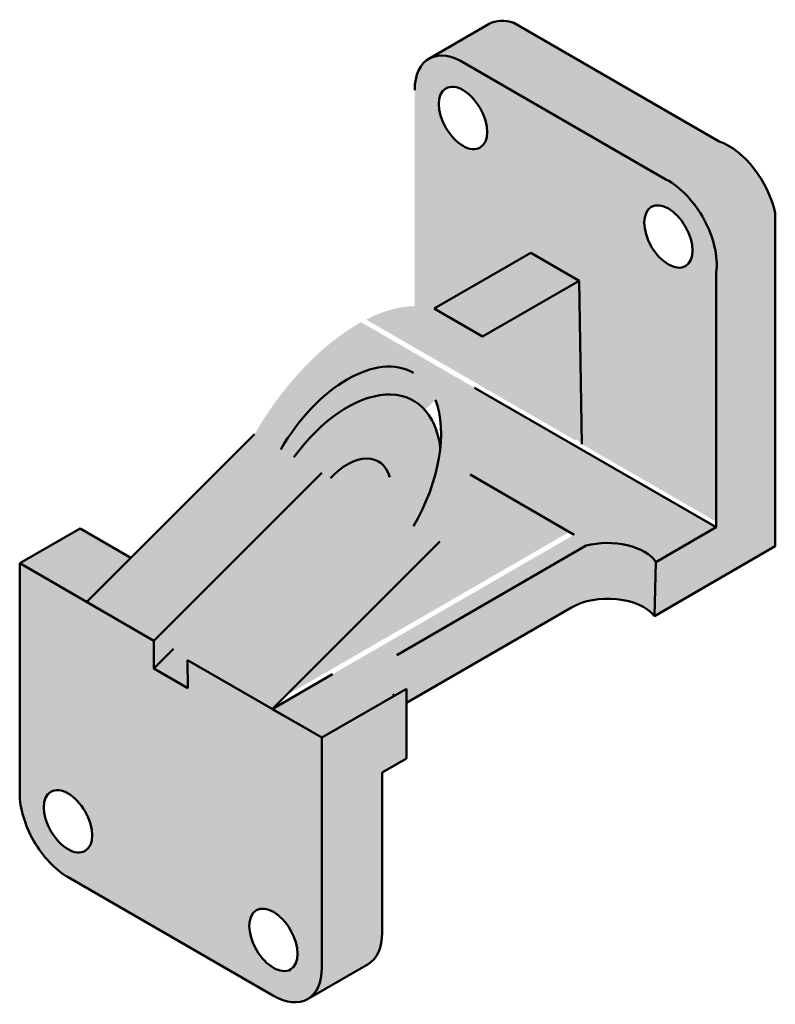
# Model space of a CAD drawing. Units: inches. Extents: x 181 to 9700, y 72 to 10161.
# Tile 1 of 2: x 181 to 452, y 72 to 425. Entities that reach past the tile are written whole.
import ezdxf

# ---------------------------------------------------------------- set-up
doc = ezdxf.new("R2010")
doc.units = ezdxf.units.IN
doc.header["$MEASUREMENT"] = 0
doc.layers.add('M-HATC', color=9, linetype='Continuous', lineweight=18)
doc.layers.add('M-OUTL', color=7, linetype='Continuous', lineweight=50)

msp = doc.modelspace()

# ---------------------------------------------------------------- hatches: boundary and pattern name
at = {"layer": 'M-HATC'}
h = msp.add_hatch(color=256, dxfattribs=at)
h.dxf.hatch_style = 1
h.paths.add_polyline_path([(289.5758214261552, 262.3998847366588), (265.5436164711371, 276.2748847366588), (205.4395400702806, 216.1708083358023), (229.4717450252987, 202.2958083358023)])
h.paths.add_polyline_path([(332.0110662115927, 237.8998847366588), (301.7001770791373, 255.3998847366588), (241.5961006782808, 195.2958083358023), (271.9069898107362, 177.7958083358023)])
edge = h.paths.add_edge_path()
edge.add_line((378.4281144762222, 241.2958083358023), (342.8085507036823, 261.8607730682951))
edge.add_ellipse((298.7773413413649, 257.0873847366588), major_axis=(-35.93948496215874, -62.24901395231655), ratio=0.5338835550983223, start_angle=450, end_angle=486.187226740073, ccw=False)
edge.add_ellipse((298.7773413413649, 257.0873847366588), major_axis=(-35.93948496215874, -62.24901395231655), ratio=0.5338835550983223, start_angle=381.6976936192442, end_angle=450, ccw=False)
edge.add_line((289.8207652336183, 195.7095837586844), (276.6390406183051, 182.5278591433712))
edge.add_line((276.6390406183051, 182.5278591433712), (291.8255740977782, 191.2958083358023))
edge.add_line((291.8255740977782, 191.2958083358023), (378.4281144762222, 241.2958083358023))
h.paths.add_polyline_path([(452.1982455472475, 236.1197151084636), (452.1982455472475, 346.5359742140326), (431.0229429833748, 334.3104075786089), (431.0229429833748, 242.9573465124921), (409.3723078887639, 230.4573465124921), (408.8969753580256, 211.1197151084636)])
edge = h.paths.add_edge_path()
edge.add_ellipse((392.1722335010851, 226.7309791545812), major_axis=(-18.37117307087383, 0), ratio=0.577350269189626, start_angle=192.224119058928, end_angle=308.65442906113)
edge.add_line((384.470166530734, 236.3604160433479), (384.470166530734, 216.3604160433479))
edge.add_ellipse((392.1722335010851, 206.7309791545811), major_axis=(-18.37117307087383, 0), ratio=0.577350269189626, start_angle=194.7034681906882, end_angle=308.65442906113003, ccw=False)
edge.add_line((408.8969753580256, 211.1197151084636), (409.3723078887639, 230.4573465124921))
edge = h.paths.add_edge_path()
edge.add_line((311.3111456829281, 155.0458083358022), (319.9713997207725, 160.0458083358023))
edge.add_line((319.9713997207725, 160.0458083358023), (319.9713997207725, 185.0458083358023))
edge.add_line((319.9713997207725, 185.0458083358023), (311.3111456829281, 180.0458083358023))
edge.add_line((311.3111456829281, 180.0458083358023), (289.6605105883172, 167.5458083358023))
edge.add_line((289.6605105883172, 167.5458083358023), (289.6605105883172, 85.04580833580225))
edge.add_ellipse((272.3400025126284, 95.04580833580229), major_axis=(12.24744871391588, -21.21320343559644), ratio=0.5773502691896262, start_angle=360.00000000000006, end_angle=390.00000000000006, ccw=False)
edge.add_line((285.6593063694593, 74.45144075550013), (306.2380863211551, 86.3326049002059))
edge.add_ellipse((293.9906376072394, 107.5458083358023), major_axis=(12.24744871391588, -21.21320343559644), ratio=0.577350269189626, start_angle=360, end_angle=390)
edge.add_line((311.3111456829281, 97.5458083358022), (311.3111456829281, 155.0458083358022))
edge = h.paths.add_edge_path()
edge.add_ellipse((361.9316820788472, 402.1604731669166), major_axis=(12.24744871391588, -21.21320343559644), ratio=0.5773502691896263, start_angle=159.0205819913284, end_angle=180)
edge.add_line((349.6842333649313, 423.3736766025129), (328.0335982703203, 410.8736766025129))
edge.add_ellipse((340.2810469842362, 389.6604731669166), major_axis=(12.24744871391588, -21.21320343559644), ratio=0.577350269189626, start_angle=152.4268374845575, end_angle=180.0000000000001, ccw=False)
edge.add_ellipse((340.2810469842362, 389.6604731669166), major_axis=(12.24744871391588, -21.21320343559644), ratio=0.577350269189626, start_angle=147.4484474656536, end_angle=152.4268374845575, ccw=False)
edge.add_line((341.1488497899605, 409.1343284863016), (413.0254035001923, 367.6363808532769))
edge.add_line((413.0254035001923, 367.6363808532769), (432.1174865026594, 381.2434445483418))
edge.add_line((432.1174865026594, 381.2434445483418), (358.5053271809825, 423.7434445483415))
edge = h.paths.add_edge_path()
edge.add_ellipse((435.5438414005244, 359.6604731669166), major_axis=(12.24744871391588, -21.21320343559644), ratio=0.577350269189626, start_angle=46.09756655575147, end_angle=159.0205819913284)
edge.add_line((432.1174865026594, 381.2434445483418), (413.0254035001923, 367.6363808532769))
edge.add_ellipse((413.8932063059135, 347.1604731669166), major_axis=(12.24744871391588, -21.21320343559644), ratio=0.5773502691896262, start_angle=37.97473599029382, end_angle=152.4268374845516, ccw=False)
edge.add_ellipse((413.8932063059135, 347.1604731669166), major_axis=(12.24744871391588, -21.21320343559644), ratio=0.5773502691896262, start_angle=23.124187939269177, end_angle=37.97473599029382, ccw=False)
edge.add_line((431.0229429833748, 334.3104075786089), (452.1982455472475, 346.5359742140326))
edge.add_line((452.1982455472475, 346.5359742140326), (452.1982455472475, 355.5381741557557))
edge = h.paths.add_edge_path()
edge.add_line((381.9139330076487, 331.3424327360183), (355.9331708941156, 316.3424327360183))
edge.add_line((355.9331708941156, 316.3424327360183), (347.2729168562712, 311.3424327360183))
edge.add_line((347.2729168562712, 311.3424327360183), (338.9373332006266, 316.1549842034574))
edge.add_ellipse((298.7773413413649, 257.0873847366588), major_axis=(-35.93948496215874, -62.24901395231655), ratio=0.5338835550983223, start_angle=516.3910297951071, end_angle=535.6085769278975)
edge.add_line((339.0824179452242, 315.9703712874247), (382.8409424408887, 272.7752374957912))
edge.add_line((382.8409424408887, 272.7752374957912), (381.9139330076487, 331.3424327360183))
edge = h.paths.add_edge_path()
edge.add_line((381.9139330076487, 331.3424327360183), (364.5934249319599, 341.3424327360183))
edge.add_line((364.5934249319599, 341.3424327360183), (338.6126628184268, 326.3424327360183))
edge.add_line((338.6126628184268, 326.3424327360183), (329.9524087805823, 321.3424327360183))
edge.add_ellipse((298.7773413413649, 257.0873847366588), major_axis=(-35.93948496215874, -62.24901395231655), ratio=0.5338835550983223, start_angle=535.8815919061803, end_angle=544.1184080938197, ccw=False)
edge.add_line((336.1655495610535, 318.417122825898), (347.2729168562712, 311.3424327360183))
edge.add_line((347.2729168562712, 311.3424327360183), (355.9331708941156, 316.3424327360183))
edge.add_line((355.9331708941156, 316.3424327360183), (381.9139330076487, 331.3424327360183))
edge = h.paths.add_edge_path()
edge.add_line((378.7961718094055, 273.1104869086883), (347.7145594960051, 291.0554641446776))
edge.add_ellipse((298.7773413413649, 257.0873847366588), major_axis=(-35.93948496215874, -62.24901395231655), ratio=0.5338835550983223, start_angle=486.187226740073, end_angle=514.7651124476778, ccw=False)
edge.add_line((342.8085507036823, 261.8607730682951), (351.059823285458, 257.0968986220499))
edge.add_line((351.059823285458, 257.0968986220499), (378.7961718094055, 273.1104869086883))
edge = h.paths.add_edge_path(flags=17)
edge.add_ellipse((298.7773413413649, 257.0873847366588), major_axis=(-35.93948496215874, -62.24901395231655), ratio=0.5338835550983223, start_angle=516.3910297951071, end_angle=535.6085769278851, ccw=False)
edge.add_line((347.6386869656112, 293.0992691705247), (380.5282226169744, 274.1104869086884))
edge.add_line((380.5282226169744, 274.1104869086884), (381.1339810930626, 274.4602217279218))
edge.add_line((381.1339810930626, 274.4602217279218), (339.0824179452354, 315.9703712874136))
h = msp.add_hatch(color=256, dxfattribs=at)
h.dxf.hatch_style = 1
edge = h.paths.add_edge_path()
edge.add_ellipse((413.8932063059135, 347.1604731669166), major_axis=(12.24744871391588, -21.21320343559644), ratio=0.5773502691896262, start_angle=37.97473599029381, end_angle=152.4268374845516)
edge.add_line((413.0254035001928, 367.6363808532767), (339.4132441785131, 410.1363808532779))
edge.add_ellipse((340.2810469842362, 389.6604731669166), major_axis=(12.24744871391588, -21.21320343559644), ratio=0.577350269189626, start_angle=152.4268374845575, end_angle=180)
edge.add_ellipse((340.2810469842362, 389.6604731669166), major_axis=(12.24744871391588, -21.21320343559644), ratio=0.577350269189626, start_angle=180, end_angle=210)
edge.add_line((322.9605389085474, 399.6604731669158), (322.9605389085474, 322.2239604497972))
edge.add_ellipse((298.7773413413649, 257.0873847366588), major_axis=(-35.93948496215874, -62.24901395231655), ratio=0.5338835550983223, start_angle=544.1184080938197, end_angle=549.6315947378079, ccw=False)
edge.add_line((329.9524087805823, 321.3424327360183), (338.6126628184268, 326.3424327360183))
edge.add_line((338.6126628184268, 326.3424327360183), (364.5934249319599, 341.3424327360183))
edge.add_line((364.5934249319599, 341.3424327360183), (381.9139330076487, 331.3424327360183))
edge.add_line((381.9139330076487, 331.3424327360183), (382.8409424408887, 272.7752374957912))
edge.add_line((382.8409424408887, 272.7752374957912), (431.0229429833748, 244.9573465124921))
edge.add_line((431.0229429833748, 244.9573465124921), (431.0229429833748, 334.3104075786089))
edge.add_ellipse((413.8932063059135, 347.1604731669166), major_axis=(12.24744871391588, -21.21320343559644), ratio=0.5773502691896262, start_angle=23.12418793926915, end_angle=37.97473599029381)
edge = h.paths.add_edge_path(flags=16)
edge.add_ellipse((413.8932063059135, 347.1604731669166), major_axis=(6.123724356957978, -10.60660171779819), ratio=0.5773502691896275, start_angle=0, end_angle=360)
edge = h.paths.add_edge_path(flags=16)
edge.add_ellipse((340.2810469842362, 389.6604731669166), major_axis=(6.123724356957978, -10.60660171779819), ratio=0.5773502691896275, start_angle=0, end_angle=360)
edge = h.paths.add_edge_path()
edge.add_line((289.6605105883172, 167.5458083358022), (241.5961006782808, 195.2958083358023))
edge.add_line((241.5961006782808, 195.2958083358023), (241.6175036323853, 185.3330109196496))
edge.add_line((241.6175036323853, 185.3330109196496), (229.4717450252987, 192.2958083358023))
edge.add_line((229.4717450252987, 192.2958083358023), (229.4717450252988, 202.2958083358023))
edge.add_line((229.4717450252988, 202.2958083358023), (181.4073351152624, 230.0458083358023))
edge.add_line((181.4073351152624, 230.0458083358023), (181.4073351152623, 147.5458083358021))
edge.add_ellipse((198.7278431909511, 137.5458083358023), major_axis=(12.24744871391588, -21.21320343559644), ratio=0.577350269189626, start_angle=210, end_angle=330.0000000000001)
edge.add_line((198.7278431909521, 117.5458083358022), (272.340002512628, 75.04580833580275))
edge.add_ellipse((272.3400025126284, 95.04580833580229), major_axis=(12.24744871391588, -21.21320343559644), ratio=0.5773502691896262, start_angle=330.0000000000001, end_angle=360)
edge.add_ellipse((272.3400025126284, 95.04580833580229), major_axis=(12.24744871391588, -21.21320343559644), ratio=0.5773502691896262, start_angle=360, end_angle=390.0000000000001)
edge.add_line((289.6605105883172, 85.04580833580206), (289.6605105883172, 167.5458083358022))
edge = h.paths.add_edge_path(flags=16)
edge.add_ellipse((272.3400025126284, 95.04580833580229), major_axis=(6.123724356957941, -10.60660171779822), ratio=0.5773502691896262, start_angle=0, end_angle=360)
edge = h.paths.add_edge_path(flags=16)
edge.add_ellipse((198.7278431909511, 137.5458083358023), major_axis=(6.123724356957941, -10.60660171779822), ratio=0.577350269189626, start_angle=0, end_angle=360)
edge = h.paths.add_edge_path()
edge.add_line((319.9713997207725, 185.0458083358023), (319.9713997207725, 180.6632076835423))
edge.add_ellipse((329.6161445207665, 189.6905531357963), major_axis=(-18.37117307087383, 0), ratio=0.5773502691896243, start_angle=403.1061845214365, end_angle=405.8946704081265)
edge.add_line((320.6448648053178, 180.4346335836542), (379.1818524443187, 214.2309791545812))
edge.add_ellipse((392.1722335010851, 206.7309791545811), major_axis=(-18.37117307087383, 0), ratio=0.577350269189626, start_angle=308.65442906113003, end_angle=330.00000000000006, ccw=False)
edge.add_line((384.470166530734, 216.3604160433479), (384.470166530734, 236.3604160433479))
edge.add_ellipse((392.1722335010851, 226.7309791545812), major_axis=(-18.37117307087383, 0), ratio=0.577350269189626, start_angle=552.224119058928, end_angle=668.65442906113, ccw=False)
edge.add_line((409.3723078887639, 230.4573465124921), (431.0229429833748, 242.9573465124921))
edge.add_line((431.0229429833748, 242.9573465124921), (381.1479140261116, 271.7527079068085))
edge.add_line((381.1479140261116, 271.7527079068085), (354.0364540342908, 255.3783400579332))
edge.add_line((354.0364540342908, 255.3783400579332), (380.160165283791, 240.2958083358022))
edge.add_line((380.160165283791, 240.2958083358022), (293.5576249053471, 190.2958083358022))
edge.add_line((293.5576249053471, 190.2958083358022), (271.9069898107361, 177.7958083358023))
edge.add_line((271.9069898107361, 177.7958083358023), (289.6605105883172, 167.5458083358023))
edge.add_line((289.6605105883172, 167.5458083358023), (311.3111456829281, 180.0458083358023))
edge.add_line((311.3111456829281, 180.0458083358023), (319.9713997207725, 185.0458083358023))
h.paths.add_polyline_path([(221.2889049756695, 232.0201732411913), (203.0579702098733, 242.5458083358023), (181.4073351152623, 230.0458083358023), (205.2230337193345, 216.2958083358023), (206.0310464212264, 216.7623146867482)])
h = msp.add_hatch(color=256, dxfattribs=at)
h.dxf.hatch_style = 1
edge = h.paths.add_edge_path(flags=17)
edge.add_ellipse((298.7773413413649, 247.0873847366588), major_axis=(-23.79589386171578, -41.21569718000821), ratio=0.5773502691896261, start_angle=156.0236431708361, end_angle=173.6492066795432)
edge.add_ellipse((298.7773413413649, 247.0873847366588), major_axis=(-23.79589386171578, -41.21569718000821), ratio=0.5773502691896261, start_angle=173.6492066795432, end_angle=252.2276840317819)
edge.add_line((279.7088665927015, 268.0965737658352), (287.5581512027334, 263.5647871832873))
edge.add_ellipse((298.7773413413649, 257.0873847366588), major_axis=(-11.21919013863152, -19.4322073398854), ratio=0.577350269189626, start_angle=494.0245231656726, end_angle=630, ccw=False)
edge.add_ellipse((298.7773413413649, 257.0873847366588), major_axis=(-11.21919013863152, -19.4322073398854), ratio=0.577350269189626, start_angle=450, end_angle=494.0245231656726, ccw=False)
edge.add_line((309.9965314799963, 250.6099822900303), (322.5732352030807, 243.3488190099894))
edge.add_ellipse((298.7773413413649, 257.0873847366588), major_axis=(-23.79589386171578, -41.21569718000821), ratio=0.5773502691896261, start_angle=450, end_angle=503.1480325575491)
edge = h.paths.add_edge_path()
edge.add_ellipse((298.7773413413649, 257.0873847366588), major_axis=(-35.93948496215874, -62.24901395231655), ratio=0.5338835550983223, start_angle=205.2348875523222, end_angle=269.9999999999999)
edge.add_line((265.5436164711371, 276.2748847366588), (274.981447479649, 270.8259504633282))
edge.add_ellipse((298.7773413413649, 257.0873847366588), major_axis=(-23.79589386171578, -41.21569718000821), ratio=0.5773502691896261, start_angle=180, end_angle=270, ccw=False)
edge.add_line((322.5732352030807, 298.303081916667), (330.3793987926145, 288.6894421879085))
edge.add_ellipse((298.7773413413649, 257.0873847366588), major_axis=(-23.79589386171578, -41.21569718000821), ratio=0.5773502691896261, start_angle=503.1480325575491, end_angle=524.9999999999999, ccw=False)
edge.add_ellipse((298.7773413413649, 257.0873847366588), major_axis=(-23.79589386171578, -41.21569718000821), ratio=0.5773502691896261, start_angle=450, end_angle=503.1480325575491, ccw=False)
edge.add_line((322.5732352030807, 243.3488190099894), (332.0110662115927, 237.8998847366588))
edge.add_ellipse((298.7773413413649, 257.0873847366588), major_axis=(-35.93948496215874, -62.24901395231655), ratio=0.5338835550983223, start_angle=450, end_angle=486.187226740073)
edge.add_ellipse((298.7773413413649, 257.0873847366588), major_axis=(-35.93948496215874, -62.24901395231655), ratio=0.5338835550983223, start_angle=486.187226740073, end_angle=514.7651124476777)
edge.add_line((347.7145594960051, 291.0554641446776), (344.420402604931, 292.9573465124921))
edge.add_line((344.420402604931, 292.9573465124921), (303.7259519491561, 316.4522985531277))
edge = h.paths.add_edge_path()
edge.add_ellipse((298.7773413413649, 257.0873847366588), major_axis=(-35.93948496215874, -62.24901395231655), ratio=0.5338835550983223, start_angle=189.6315947378079, end_angle=203.6089702048929)
edge.add_line((305.533875287119, 317.4084935272806), (322.9605389085474, 307.3472045943719))
edge.add_line((322.9605389085474, 307.3472045943719), (322.9605389085474, 322.2239604497972))
edge = h.paths.add_edge_path()
edge.add_line((339.0824179452244, 315.9703712874247), (338.8363115105899, 316.213309103394))
edge.add_line((338.8363115105899, 316.213309103394), (329.9524087805823, 321.3424327360183))
edge.add_ellipse((298.7773413413649, 257.0873847366588), major_axis=(-35.93948496215874, -62.24901395231655), ratio=0.5338835550983223, start_angle=184.1184080938196, end_angle=189.6315947378079)
edge.add_line((322.9605389085474, 322.2239604497972), (322.9605389085474, 307.3472045943719))
edge.add_line((322.9605389085474, 307.3472045943719), (347.6386869656112, 293.0992691705247))
edge.add_ellipse((298.7773413413649, 257.0873847366588), major_axis=(-35.93948496215874, -62.24901395231655), ratio=0.5338835550983223, start_angle=516.3910297951071, end_angle=535.6085769278975)
edge = h.paths.add_edge_path(flags=17)
edge.add_ellipse((298.7773413413649, 257.0873847366588), major_axis=(-23.79589386171578, -41.21569718000821), ratio=0.5773502691896261, start_angle=180, end_angle=270)
edge.add_line((274.981447479649, 270.8259504633282), (279.7088665927015, 268.0965737658352))
edge.add_ellipse((298.7773413413649, 247.0873847366588), major_axis=(-23.79589386171578, -41.21569718000821), ratio=0.5773502691896261, start_angle=173.6492066795432, end_angle=252.22768403178202, ccw=False)
edge.add_line((326.6473484853686, 284.9573918806626), (330.3793987926145, 288.6894421879085))
edge.add_line((330.3793987926145, 288.6894421879085), (322.5732352030807, 298.303081916667))
edge = h.paths.add_edge_path(flags=16)
edge.add_ellipse((298.7773413413649, 257.0873847366588), major_axis=(-11.21919013863152, -19.4322073398854), ratio=0.577350269189626, start_angle=494.0245231656725, end_angle=269.9999999999999)
edge.add_line((287.5581512027334, 263.5647871832873), (292.7575781499145, 260.5628966357005))
edge.add_ellipse((298.7773413413649, 247.0873847366588), major_axis=(-11.21919013863152, -19.4322073398854), ratio=0.577350269189626, start_angle=183.4370999248528, end_angle=234.0712087957403, ccw=False)
edge.add_ellipse((298.7773413413649, 247.0873847366588), major_axis=(-11.21919013863152, -19.4322073398854), ratio=0.577350269189626, start_angle=162.1425081607802, end_angle=183.4370999248528, ccw=False)
h.paths.add_polyline_path([(295.9155673883109, 258.7396306988144), (289.5758214261552, 262.3998847366588), (229.4717450252987, 202.2958083358024), (229.4717450252987, 192.2958083358023), (236.5428128371642, 199.3668761476677)])
h.paths.add_polyline_path([(301.7001770791373, 255.3998847366588), (295.9155673883109, 258.7396306988144), (236.5428128371642, 199.3668761476677), (229.4717450252987, 192.2958083358023), (241.6175036323853, 185.3330109196496), (241.5961006782808, 195.2958083358023)])
edge = h.paths.add_edge_path(flags=16)
edge.add_ellipse((298.7773413413649, 247.0873847366588), major_axis=(-11.21919013863152, -19.4322073398854), ratio=0.577350269189626, start_angle=162.1425081607801, end_angle=183.4370999248528)
edge.add_line((308.7754643622091, 267.085507757503), (298.7773413413649, 257.0873847366588))
edge.add_line((298.7773413413649, 257.0873847366588), (301.7001770791373, 255.3998847366588))
edge.add_line((301.7001770791373, 255.3998847366588), (309.9965314799963, 250.6099822900304))
edge.add_ellipse((298.7773413413649, 257.0873847366588), major_axis=(-11.21919013863152, -19.4322073398854), ratio=0.577350269189626, start_angle=450, end_angle=494.0245231656725)
edge = h.paths.add_edge_path(flags=16)
edge.add_ellipse((298.7773413413649, 247.0873847366588), major_axis=(-11.21919013863152, -19.4322073398854), ratio=0.577350269189626, start_angle=183.4370999248528, end_angle=234.0712087957403)
edge.add_line((292.7575781499145, 260.5628966357005), (295.9155673883109, 258.7396306988144))
edge.add_line((295.9155673883109, 258.7396306988144), (298.7773413413649, 257.0873847366588))
edge.add_line((298.7773413413649, 257.0873847366588), (308.775464362209, 267.085507757503))
edge = h.paths.add_edge_path()
edge.add_ellipse((298.7773413413649, 257.0873847366588), major_axis=(-35.93948496215874, -62.24901395231655), ratio=0.5338835550983223, start_angle=381.6976936192442, end_angle=450)
edge.add_line((332.0110662115928, 237.8998847366589), (289.8207652336182, 195.7095837586843))
h.paths.add_polyline_path([(381.1479140261116, 271.7527079068085), (378.7961718094055, 273.1104869086883), (351.059823285458, 257.0968986220499), (354.0364540342908, 255.3783400579332)])

# ---------------------------------------------------------------- linework, layer by layer
at = {"layer": 'M-OUTL'}
for p, q in [((432.1174865026594, 381.2434445483418), (358.5053271809823, 423.7434445483417)), ((349.6842333649313, 423.373676602513), (328.0335982703203, 410.873676602513)), ((413.0254035001916, 367.6363808532773), (339.4132441785136, 410.1363808532775)), ((401.6457575919976, 368.3736766025131), (401.6457575919976, 368.3736766025131)), ((452.1982455472475, 236.1197151084636), (452.1982455472475, 355.5381741557557)), ((338.6126628184268, 326.3424327360183), (364.5934249319599, 341.3424327360183)), ((364.5934249319599, 341.3424327360183), (381.9139330076487, 331.3424327360183)), ((431.0229429833748, 340.2308225914648), (431.0229429833748, 340.4573465124921)), ((431.0229429833748, 242.9573465124921), (431.0229429833748, 334.3104075786089)), ((381.9139330076487, 331.3424327360183), (355.9331708941156, 316.3424327360183)), ((381.9139330076487, 331.3424327360183), (382.8409424408887, 272.7752374957912)), ((329.9524087805824, 321.3424327360183), (338.6126628184268, 326.3424327360183)), ((347.2729168562712, 311.3424327360183), (329.9524087805823, 321.3424327360183)), ((355.9331708941156, 316.3424327360183), (347.2729168562712, 311.3424327360183)), ((431.0229429833748, 242.9573465124921), (344.420402604931, 292.9573465124921)), ((205.4395400702806, 216.1708083358023), (265.5436164711371, 276.2748847366588)), ((229.4717450252987, 202.2958083358023), (289.6605105883172, 262.4845738988208)), ((380.160165283791, 240.2958083358023), (342.8085507036823, 261.8607730682951)), ((431.0229429833748, 242.9573465124921), (431.0229429833748, 244.9573465124921)), ((181.4073351152623, 230.0458083358023), (203.0579702098733, 242.5458083358023)), ((203.0579702098733, 242.5458083358023), (221.2889049756695, 232.0201732411913)), ((409.3723078887639, 230.4573465124921), (431.0229429833748, 242.9573465124921)), ((271.9069898107362, 177.7958083358023), (332.0110662115927, 237.8998847366588)), ((316.5735907955658, 197.1603097655947), (384.470166530734, 236.3604160433479)), ((408.8969753580256, 211.1197151084636), (452.1982455472475, 236.1197151084636)), ((181.4073351152623, 147.5458083358023), (181.4073351152623, 230.0458083358023)), ((181.4073351152623, 230.0458083358023), (229.4717450252987, 202.2958083358023)), ((408.8969753580256, 211.1197151084636), (409.3723078887639, 230.4573465124921)), ((205.2230337193345, 216.2958083358023), (206.0310464212266, 216.7623146867483)), ((205.4395400702805, 216.1708083358023), (205.2230337193345, 216.2958083358023)), ((205.4395400702806, 216.1708083358023), (205.2230337193345, 216.2958083358024)), ((205.4395400702805, 216.1708083358023), (205.2230337193345, 216.2958083358023)), ((384.470166530734, 216.3604160433479), (384.4701665307341, 216.360416043348)), ((319.9713997207725, 180.0458083358022), (379.1818524443185, 214.2309791545811)), ((229.4717450252987, 202.2958083358023), (229.4717450252987, 192.2958083358023)), ((229.4717450252987, 192.2958083358023), (236.5428128371642, 199.3668761476677)), ((235.5339228517898, 198.7958083358023), (235.8114909874544, 198.6355542979579)), ((241.5961006782808, 195.2958083358023), (289.6605105883172, 167.5458083358023)), ((241.6175036323853, 185.3330109196496), (241.5961006782808, 195.2958083358023)), ((229.4717450252987, 192.2958083358023), (241.6175036323853, 185.3330109196496)), ((271.9069898107362, 177.7958083358023), (293.5576249053472, 190.2958083358022)), ((311.3111456829281, 180.0458083358023), (319.9713997207726, 185.0458083358023)), ((319.9713997207725, 185.0458083358023), (319.9713997207725, 160.0458083358023)), ((311.3111456829281, 180.0458083358023), (289.6605105883172, 167.5458083358023)), ((271.9069898107363, 177.7958083358023), (285.330383569395, 170.0458083358023)), ((289.6605105883172, 85.04580833580229), (289.6605105883172, 167.5458083358023)), ((319.9713997207725, 160.0458083358023), (311.3111456829281, 155.0458083358023)), ((311.3111456829281, 97.54580833580229), (311.3111456829281, 155.0458083358023)), ((272.3400025126284, 75.04580833580229), (198.7278431909511, 117.5458083358023)), ((284.5874512265443, 73.83260490020587), (306.2380863211553, 86.33260490020585)), ((306.2380863211553, 86.33260490020585), (306.2380863212561, 86.33260490026412))]:
    msp.add_line(p, q, dxfattribs=at)
for centre, major_axis, ratio, start_param, end_param in [((361.9316820788472, 402.1604731669166), (12.24744871391588, -21.21320343559644), 0.5773502691896262, 2.555328667204451, 3.141592653589793), ((340.2810469842362, 389.6604731669166), (12.24744871391588, -21.21320343559644), 0.5773502691896262, 2.306070886259445, 3.926990816987241), ((435.5438414005244, 359.6604731669166), (12.24744871391588, -21.21320343559644), 0.5773502691896262, 1.063630385740387, 2.555328667204451), ((413.8932063059135, 347.1604731669166), (12.24744871391588, -21.21320343559644), 0.5773502691896262, 0.6368419777653243, 2.406318094125164), ((298.7773413413649, 257.0873847366588), (-23.79589386171578, -41.21569718000821), 0.5773502691896261, 3.141592653589793, 4.712388980384689), ((298.7773413413649, 247.0873847366588), (-23.79589386171578, -41.21569718000821), 0.5773502691896261, 2.485224090838563, 4.52939995338473), ((298.7773413413649, 257.0873847366588), (-23.79589386171578, -41.21569718000821), 0.5773502691896261, 7.853981633974482, 8.990259208244188), ((298.7773413413649, 247.0873847366588), (-11.21919013863152, -19.4322073398854), 0.577350269189626, 2.632614110461153, 4.316143805025259), ((392.1722335010851, 226.7309791545812), (-18.37117307087383, 0), 0.577350269189626, 9.7837642072565, 11.42819050285597), ((392.1722335010851, 206.7309791545811), (-18.37117307087383, 0), 0.577350269189626, 3.568188346063852, 5.497787143782139), ((332.2004461011292, 187.1062515554336), (-18.37117307087383, 0), 0.577350269189626, 6.665644395551503, 6.728746561122909), ((329.6161445207665, 189.6905531357963), (-18.37117307087383, 0), 0.5773502691896243, 7.301274263515839, 7.343801311630352), ((198.7278431909511, 137.5458083358023), (12.24744871391588, -21.21320343559644), 0.5773502691896262, 3.926990816987241, 5.49778714378214), ((293.9906376072394, 107.5458083358023), (12.24744871391588, -21.21320343559644), 0.5773502691896262, 6.283185307179586, 7.068583470577035), ((272.3400025126284, 95.04580833580229), (12.24744871391588, -21.21320343559644), 0.5773502691896262, 5.497787143782138, 7.068583470577035)]:
    msp.add_ellipse(centre, major_axis=major_axis, ratio=ratio, start_param=start_param, end_param=end_param, dxfattribs=at)
for centre, major_axis, ratio in [((340.2810469842362, 389.6604731669166), (6.123724356957978, -10.60660171779819), 0.5773502691896275), ((413.8932063059135, 347.1604731669166), (6.123724356957978, -10.60660171779819), 0.5773502691896275), ((198.7278431909511, 137.5458083358023), (6.123724356957941, -10.60660171779822), 0.5773502691896262), ((272.3400025126284, 95.04580833580229), (6.123724356957941, -10.60660171779822), 0.5773502691896262)]:
    msp.add_ellipse(centre, major_axis=major_axis, ratio=ratio, dxfattribs=at)

doc.saveas('drawing.dxf')
